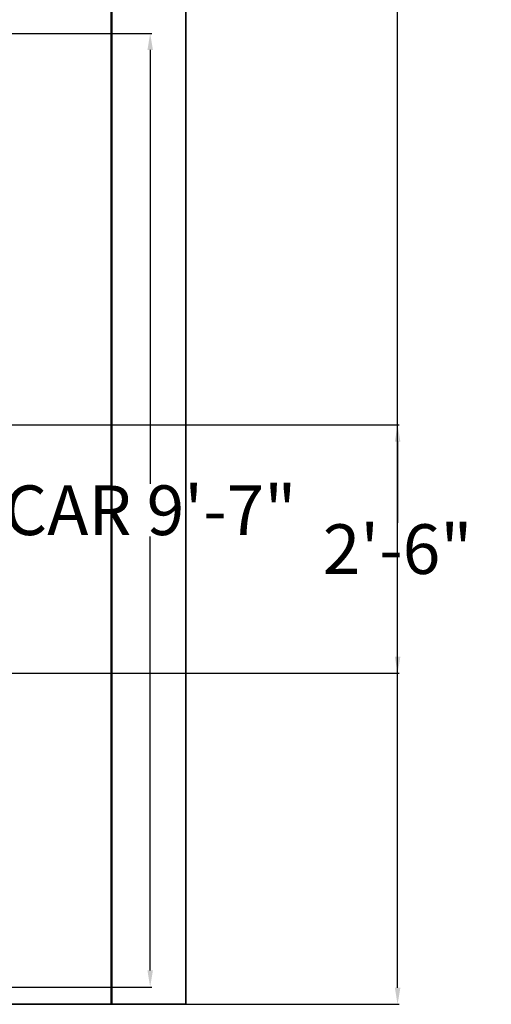
# Model space of a CAD drawing. Units: inches. Extents: x 134 to 568, y 15 to 554.
# Tile 4 of 7: x 511 to 568, y 45 to 164. Entities that reach past the tile are written whole.
import ezdxf

# ---------------------------------------------------------------- set-up
doc = ezdxf.new("R2010")
doc.units = ezdxf.units.IN
doc.header["$MEASUREMENT"] = 0
for name, color, linetype, lineweight in [('A-ANNO-DIMS', 2, 'Continuous', 18), ('A-WALL', 7, 'Continuous', 50), ('C-PROP', 7, 'Continuous', 35)]:
    doc.layers.add(name, color=color, linetype=linetype, lineweight=lineweight)
doc.styles.get("Standard").update_dxf_attribs({"font": 'arial.ttf'})
doc.dimstyles.get("Standard").update_dxf_attribs({"dimtxt": 6, "dimasz": 2, "dimexe": 0.18, "dimexo": 0.0625, "dimgap": 0.09, "dimtad": 0, "dimtih": 1, "dimtoh": 1, "dimdec": 0, "dimzin": 0, "dimdsep": 46, "dimlunit": 4, "dimtxsty": 'Standard', "dimcen": 0.09, "dimadec": 0, "dimazin": 0, "dimtfac": 1, "dimtdec": 0, "dimtofl": 0, "dimtmove": 0, "dimatfit": 3, "dimfxl": 1, "dimtolj": 1, "dimtzin": 0, "dimarcsym": 0})

# ---------------------------------------------------------------- blocks, each defined once
blk = doc.blocks.new('*D2')
at = {"layer": 'A-ANNO-DIMS', "color": 0, "lineweight": -2, "transparency": 16777216}
for p, q in [((457.08, 190.52), (457.08, 165.33)), ((522.08, 190.52), (522.08, 165.33)), ((459.08, 165.51), (481.52, 165.51)), ((520.08, 165.51), (497.65, 165.51))]:
    blk.add_line(p, q, dxfattribs=at)
at = {"layer": 'A-ANNO-DIMS', "color": 0, "transparency": 16777216}
for points in [[(459.08, 165.84), (459.08, 165.18), (457.08, 165.51)], [(520.08, 165.84), (520.08, 165.18), (522.08, 165.51)]]:
    blk.add_solid(points, dxfattribs=at)
at = {"layer": 'Defpoints', "color": 0, "transparency": 16777216}
for p in [(457.08, 190.58), (522.08, 190.58), (522.08, 165.51)]:
    blk.add_point(p, dxfattribs=at)
at = {"layer": 'A-ANNO-DIMS', "color": 0, "transparency": 16777216, "insert": (489.58, 165.51), "char_height": 6, "attachment_point": 5}
blk.add_mtext('\\A1;5\'-5"', dxfattribs=at)
blk = doc.blocks.new('*D6')
at = {"layer": 'A-ANNO-DIMS', "color": 0, "lineweight": -2, "transparency": 16777216}
for p, q in [((522.02, 190.58), (439.72, 190.58)), ((439.9, 188.58), (439.9, 120.68)), ((439.9, 46.58), (439.9, 114.48)), ((522.02, 44.58), (439.72, 44.58))]:
    blk.add_line(p, q, dxfattribs=at)
at = {"layer": 'A-ANNO-DIMS', "color": 0, "transparency": 16777216}
for points in [[(439.57, 188.58), (440.23, 188.58), (439.9, 190.58)], [(439.57, 46.58), (440.23, 46.58), (439.9, 44.58)]]:
    blk.add_solid(points, dxfattribs=at)
at = {"layer": 'Defpoints', "color": 0, "transparency": 16777216}
for p in [(439.9, 190.58), (522.08, 190.58), (522.08, 44.58)]:
    blk.add_point(p, dxfattribs=at)
at = {"layer": 'A-ANNO-DIMS', "color": 0, "transparency": 16777216, "insert": (439.9, 117.58), "char_height": 6, "attachment_point": 5}
blk.add_mtext('\\A1;12\'-2"', dxfattribs=at)
blk = doc.blocks.new('*D56')
at = {"layer": 'A-ANNO-DIMS', "color": 0, "lineweight": -2, "transparency": 16777216}
for p, q in [((509.54, 161.9), (526.94, 161.9)), ((526.76, 159.9), (526.76, 107.47)), ((526.76, 48.67), (526.76, 101.09)), ((509.54, 46.67), (526.94, 46.67))]:
    blk.add_line(p, q, dxfattribs=at)
at = {"layer": 'A-ANNO-DIMS', "color": 0, "transparency": 16777216}
for points in [[(526.43, 159.9), (527.09, 159.9), (526.76, 161.9)], [(526.43, 48.67), (527.09, 48.67), (526.76, 46.67)]]:
    blk.add_solid(points, dxfattribs=at)
at = {"layer": 'Defpoints', "color": 0, "transparency": 16777216}
for p in [(509.48, 161.9), (526.76, 161.9), (509.48, 46.67)]:
    blk.add_point(p, dxfattribs=at)
at = {"layer": 'A-ANNO-DIMS', "color": 0, "transparency": 16777216, "insert": (526.76, 104.28), "char_height": 6, "attachment_point": 5}
blk.add_mtext('\\A1;CAR 9\'-7"', dxfattribs=at)
blk = doc.blocks.new('*D60')
at = {"layer": 'A-ANNO-DIMS', "color": 0, "lineweight": -2, "transparency": 16777216}
for p, q in [((522.15, 515.58), (556.81, 515.58)), ((556.63, 513.58), (556.63, 283.24)), ((556.63, 46.58), (556.63, 276.93)), ((522.15, 44.58), (556.81, 44.58))]:
    blk.add_line(p, q, dxfattribs=at)
at = {"layer": 'A-ANNO-DIMS', "color": 0, "transparency": 16777216}
for points in [[(556.3, 513.58), (556.97, 513.58), (556.63, 515.58)], [(556.3, 46.58), (556.97, 46.58), (556.63, 44.58)]]:
    blk.add_solid(points, dxfattribs=at)
at = {"layer": 'Defpoints', "color": 0, "transparency": 16777216}
for p in [(522.08, 515.58), (556.63, 515.58), (522.08, 44.58)]:
    blk.add_point(p, dxfattribs=at)
at = {"layer": 'A-ANNO-DIMS', "color": 0, "transparency": 16777216, "insert": (556.63, 280.08), "char_height": 6, "attachment_point": 5}
blk.add_mtext('\\A1;39\'-3"', dxfattribs=at)
blk = doc.blocks.new('*D62')
at = {"layer": 'A-ANNO-DIMS', "color": 0, "lineweight": -2, "transparency": 16777216}
for p, q in [((346.65, 114.58), (556.81, 114.58)), ((556.63, 112.58), (556.63, 102.74)), ((556.63, 86.58), (556.63, 96.43)), ((346.65, 84.58), (556.81, 84.58))]:
    blk.add_line(p, q, dxfattribs=at)
at = {"layer": 'A-ANNO-DIMS', "color": 0, "transparency": 16777216}
for points in [[(556.3, 112.58), (556.97, 112.58), (556.63, 114.58)], [(556.3, 86.58), (556.97, 86.58), (556.63, 84.58)]]:
    blk.add_solid(points, dxfattribs=at)
at = {"layer": 'Defpoints', "color": 0, "transparency": 16777216}
for p in [(346.58, 114.58), (556.63, 114.58), (346.58, 84.58)]:
    blk.add_point(p, dxfattribs=at)
at = {"layer": 'A-ANNO-DIMS', "color": 0, "transparency": 16777216, "insert": (556.63, 99.58), "char_height": 6, "attachment_point": 5}
blk.add_mtext('\\A1;2\'-6"', dxfattribs=at)

msp = doc.modelspace()

# ---------------------------------------------------------------- linework, layer by layer
at = {"layer": 'A-WALL'}
msp.add_line((522.08, 44.58), (522.08, 230.58), dxfattribs=at)
at = {"layer": 'C-PROP'}
for p, q in [((531.08, 44.58), (531.08, 524.58)), ((171.08, 44.58), (531.08, 44.58))]:
    msp.add_line(p, q, dxfattribs=at)

# ---------------------------------------------------------------- dimensions: what is measured, and where the dimension line sits
at = {"layer": 'A-ANNO-DIMS'}
for base, p1, p2, override, picture, middle in [((556.63, 515.58), (522.08, 44.58), (522.08, 515.58), {"dimdec": 1, "dimlfac": 1, "dimrnd": 0, "dimzin": 1, "dimdsep": 46, "dimlunit": 4, "dimfrac": 2}, '*D60', (556.63, 280.08)), ((439.9, 190.58), (522.08, 44.58), (522.08, 190.58), {"dimclrd": 0, "dimclre": 0, "dimclrt": 0}, '*D6', (439.9, 117.58)), ((556.63, 114.58), (346.58, 84.58), (346.58, 114.58), {"dimdec": 1, "dimlfac": 1, "dimrnd": 0, "dimzin": 1, "dimdsep": 46, "dimlunit": 4, "dimfrac": 2}, '*D62', (556.63, 99.58))]:
    dim = msp.add_linear_dim(base=base, p1=p1, p2=p2, angle=90, dimstyle='Standard', override=override, dxfattribs=at)
    dim.commit()
    dim.dimension.update_dxf_attribs({"geometry": picture, "text_midpoint": middle})
dim = msp.add_linear_dim(base=(522.08, 165.51), p1=(457.08, 190.58), p2=(522.08, 190.58), dimstyle='Standard', override={"dimclrd": 0, "dimclre": 0, "dimclrt": 0}, dxfattribs=at)
dim.commit()
dim.dimension.update_dxf_attribs({"geometry": '*D2', "text_midpoint": (489.58, 165.51)})
dim = msp.add_linear_dim(base=(526.76, 161.9), p1=(509.48, 46.67), p2=(509.48, 161.9), angle=90, text='CAR <>', dimstyle='Standard', override={"dimdec": 1, "dimlfac": 1, "dimrnd": 0, "dimzin": 1, "dimdsep": 46, "dimlunit": 4, "dimfrac": 2}, dxfattribs=at)
dim.commit()
dim.dimension.update_dxf_attribs({"geometry": '*D56', "text_midpoint": (526.76, 104.28)})

doc.saveas('drawing.dxf')
